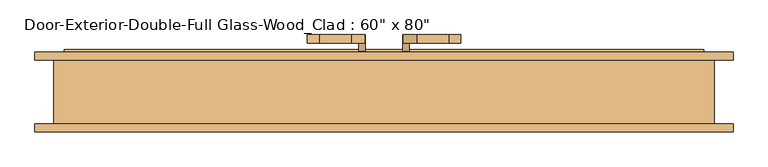
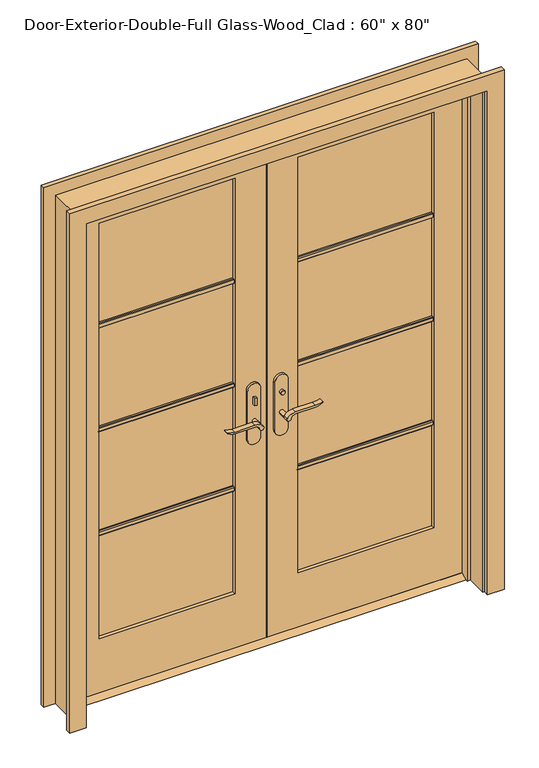
"""IFC4 building model written with IfcOpenShell, lengths in millimetres: door geometry."""

from ifc_helpers import new_model, si_unit, point, frame, frame_2d, origin, place, context, project, spatial, polyline, circle_curve, trimmed, segment, composite_curve, outline, extrude, faceted_brep, source, transform, mapped, element, save


def door_94998e6c(model_context):
    return source(origin(), model_context, "Body", "SolidModel", [
        extrude(outline(polyline([(38.1, 12.7), (73.025, 12.7), (98.425, 0.0), (12.7, 0.0), (38.1, 12.7)])), frame((-762.0, 0.0, 0.0), z_axis=(1.0, 0.0, 0.0), x_axis=(0.0, 1.0, 0.0)), (0.0, 0.0, 1.0), 1524.0),
        extrude(outline(polyline([(-47.4019111, 18.1), (-57.4019111, 18.1), (-57.4019111, 28.1), (-47.4019111, 28.1), (-47.4019111, 18.1)])), frame((0.0, 0.0, 981.9), z_axis=(0.0, 0.0, 1.0), x_axis=(1.0, 0.0, 0.0)), (0.0, 0.0, 1.0), 30.0),
        extrude(outline(composite_curve([segment(trimmed(circle_curve(frame_2d((996.9, -52.4019111)), 8.0), [point((996.9, -60.4019111))], [point((996.9, -44.4019111))], False, "CARTESIAN"), True, "CONTINUOUS"), segment(trimmed(circle_curve(frame_2d((996.9, -52.4019111)), 8.0), [point((996.9, -44.4019111))], [point((996.9, -60.4019111))], False, "CARTESIAN"), True, "CONTINUOUS")], self_intersect=False)), frame((0.0, 83.025, 0.0), z_axis=(0.0, 1.0, 0.0), x_axis=(0.0, 0.0, 1.0)), (0.0, 0.0, 1.0), 10.0),
        extrude(outline(composite_curve([segment(trimmed(circle_curve(frame_2d((897.1555521, -76.0694241)), 37.2832219), [point((919.0523287, -45.8937749))], [point((934.4, -77.7693445))], False, "CARTESIAN"), True, "CONTINUOUS"), segment(polyline([(934.4, -77.7693445), (934.4, -154.045502)]), True, "CONTINUOUS"), segment(trimmed(circle_curve(frame_2d((1017.6850638, -153.9791202)), 83.2850902), [point((934.4, -154.045502))], [point((939.4, -182.4019111))], True, "CARTESIAN"), True, "CONTINUOUS"), segment(polyline([(939.4, -182.4019111), (936.6135558, -182.4019111)]), True, "CONTINUOUS"), segment(trimmed(circle_curve(frame_2d((986.6709207, -150.4622499)), 59.3791355), [point((936.6135558, -182.4019111))], [point((927.4, -154.045502))], False, "CARTESIAN"), True, "CONTINUOUS"), segment(polyline([(927.4, -154.045502), (927.4, -77.7881013)]), True, "CONTINUOUS"), segment(trimmed(circle_curve(frame_2d((909.2738613, -77.7881013)), 18.1261387), [point((927.4, -77.7881013))], [point((914.4, -60.4019111))], True, "CARTESIAN"), True, "CONTINUOUS"), segment(trimmed(circle_curve(frame_2d((914.4, -52.4019111)), 8.0), [point((914.4, -60.4019111))], [point((919.0523287, -45.8937749))], False, "CARTESIAN"), True, "CONTINUOUS")], self_intersect=False)), frame((0.0, -21.9, 0.0), z_axis=(0.0, 1.0, 0.0), x_axis=(0.0, 0.0, 1.0)), (0.0, 0.0, 1.0), 20.0),
        extrude(outline(composite_curve([segment(trimmed(circle_curve(frame_2d((914.4, -52.4019111)), 8.0), [point((914.3999903, -60.4019111))], [point((919.0523287, -45.8937749))], False, "CARTESIAN"), True, "CONTINUOUS"), segment(trimmed(circle_curve(frame_2d((897.1555521, -76.0694241)), 37.2832219), [point((919.0523287, -45.8937749))], [point((934.4, -77.7693445))], False, "CARTESIAN"), True, "CONTINUOUS"), segment(polyline([(934.4, -77.7693445), (934.4, -154.045502)]), True, "CONTINUOUS"), segment(trimmed(circle_curve(frame_2d((1017.6850638, -153.9791202)), 83.2850902), [point((934.4, -154.045502))], [point((939.4, -182.4019111))], True, "CARTESIAN"), True, "CONTINUOUS"), segment(polyline([(939.4, -182.4019111), (936.6135558, -182.4019111)]), True, "CONTINUOUS"), segment(trimmed(circle_curve(frame_2d((986.6709207, -150.4622499)), 59.3791355), [point((936.6135558, -182.4019111))], [point((927.4, -154.045502))], False, "CARTESIAN"), True, "CONTINUOUS"), segment(polyline([(927.4, -154.045502), (927.4, -77.788099)]), True, "CONTINUOUS"), segment(trimmed(circle_curve(frame_2d((909.2738682, -77.788099)), 18.1261318), [point((927.4, -77.788099))], [point((914.3999903, -60.4019111))], True, "CARTESIAN"), True, "CONTINUOUS")], self_intersect=False)), frame((0.0, 113.025, 0.0), z_axis=(0.0, 1.0, 0.0), x_axis=(0.0, 0.0, 1.0)), (0.0, 0.0, 1.0), 20.0),
        extrude(outline(composite_curve([segment(trimmed(circle_curve(frame_2d((914.4, -52.4019111)), 8.0), [point((914.4, -60.4019111))], [point((914.4, -44.4019111))], False, "CARTESIAN"), True, "CONTINUOUS"), segment(trimmed(circle_curve(frame_2d((914.4, -52.4019111)), 8.0), [point((914.4, -44.4019111))], [point((914.4, -60.4019111))], False, "CARTESIAN"), True, "CONTINUOUS")], self_intersect=False)), frame((0.0, -1.9, 0.0), z_axis=(0.0, 1.0, 0.0), x_axis=(0.0, 0.0, 1.0)), (0.0, 0.0, 1.0), 30.0),
        extrude(outline(composite_curve([segment(trimmed(circle_curve(frame_2d((914.4, -52.4019111)), 8.0), [point((914.4, -60.4019111))], [point((914.4, -44.4019111))], False, "CARTESIAN"), True, "CONTINUOUS"), segment(trimmed(circle_curve(frame_2d((914.4, -52.4019111)), 8.0), [point((914.4, -44.4019111))], [point((914.4, -60.4019111))], False, "CARTESIAN"), True, "CONTINUOUS")], self_intersect=False)), frame((0.0, 83.025, 0.0), z_axis=(0.0, 1.0, 0.0), x_axis=(0.0, 0.0, 1.0)), (0.0, 0.0, 1.0), 30.0),
        extrude(outline(composite_curve([segment(polyline([(844.4, -27.4019111), (1039.4, -27.4019111)]), True, "CONTINUOUS"), segment(trimmed(circle_curve(frame_2d((1039.4, -52.4019111)), 25.0), [point((1039.4, -27.4019111))], [point((1039.4, -77.4019111))], False, "CARTESIAN"), True, "CONTINUOUS"), segment(polyline([(1039.4, -77.4019111), (844.4, -77.4019111)]), True, "CONTINUOUS"), segment(trimmed(circle_curve(frame_2d((844.4, -52.4019111)), 25.0), [point((844.4, -77.4019111))], [point((844.4, -27.4019111))], False, "CARTESIAN"), True, "CONTINUOUS")], self_intersect=False)), frame((0.0, 28.1, 0.0), z_axis=(0.0, 1.0, 0.0), x_axis=(0.0, 0.0, 1.0)), (0.0, 0.0, 1.0), 10.0),
        extrude(outline(composite_curve([segment(polyline([(844.4, -27.4019111), (1039.4, -27.4019111)]), True, "CONTINUOUS"), segment(trimmed(circle_curve(frame_2d((1039.4, -52.4019111)), 25.0), [point((1039.4, -27.4019111))], [point((1039.4, -77.4019111))], False, "CARTESIAN"), True, "CONTINUOUS"), segment(polyline([(1039.4, -77.4019111), (844.4, -77.4019111)]), True, "CONTINUOUS"), segment(trimmed(circle_curve(frame_2d((844.4, -52.4019111)), 25.0), [point((844.4, -77.4019111))], [point((844.4, -27.4019111))], False, "CARTESIAN"), True, "CONTINUOUS")], self_intersect=False)), frame((0.0, 73.025, 0.0), z_axis=(0.0, 1.0, 0.0), x_axis=(0.0, 0.0, 1.0)), (0.0, 0.0, 1.0), 10.0),
        extrude(outline(polyline([(47.3875, 93.025), (57.3875, 93.025), (57.3875, 83.025), (47.3875, 83.025), (47.3875, 93.025)])), frame((0.0, 0.0, 981.9), z_axis=(0.0, 0.0, 1.0), x_axis=(1.0, 0.0, 0.0)), (0.0, 0.0, 1.0), 30.0),
        extrude(outline(composite_curve([segment(trimmed(circle_curve(frame_2d((996.9, 52.3875)), 8.0), [point((996.9, 60.3875))], [point((996.9, 44.3875))], False, "CARTESIAN"), True, "CONTINUOUS"), segment(trimmed(circle_curve(frame_2d((996.9, 52.3875)), 8.0), [point((996.9, 44.3875))], [point((996.9, 60.3875))], False, "CARTESIAN"), True, "CONTINUOUS")], self_intersect=False)), frame((0.0, 18.1, 0.0), z_axis=(0.0, 1.0, 0.0), x_axis=(0.0, 0.0, 1.0)), (0.0, 0.0, 1.0), 10.0),
        extrude(outline(composite_curve([segment(trimmed(circle_curve(frame_2d((914.4, 52.3875)), 8.0), [point((919.0523287, 45.8793637))], [point((914.4, 60.3875))], False, "CARTESIAN"), True, "CONTINUOUS"), segment(trimmed(circle_curve(frame_2d((909.2738613, 77.7736901)), 18.1261387), [point((914.4, 60.3875))], [point((927.4, 77.7736901))], True, "CARTESIAN"), True, "CONTINUOUS"), segment(polyline([(927.4, 77.7736901), (927.4, 154.0310909)]), True, "CONTINUOUS"), segment(trimmed(circle_curve(frame_2d((986.6709207, 150.4478388)), 59.3791355), [point((927.4, 154.0310909))], [point((936.6135558, 182.3875))], False, "CARTESIAN"), True, "CONTINUOUS"), segment(polyline([(936.6135558, 182.3875), (939.4, 182.3875)]), True, "CONTINUOUS"), segment(trimmed(circle_curve(frame_2d((1017.6850638, 153.9647091)), 83.2850902), [point((939.4, 182.3875))], [point((934.4, 154.0310909))], True, "CARTESIAN"), True, "CONTINUOUS"), segment(polyline([(934.4, 154.0310909), (934.4, 77.7549333)]), True, "CONTINUOUS"), segment(trimmed(circle_curve(frame_2d((897.1555521, 76.0550129)), 37.2832219), [point((934.4, 77.7549333))], [point((919.0523287, 45.8793637))], False, "CARTESIAN"), True, "CONTINUOUS")], self_intersect=False)), frame((0.0, 113.025, 0.0), z_axis=(0.0, 1.0, 0.0), x_axis=(0.0, 0.0, 1.0)), (0.0, 0.0, 1.0), 20.0),
        extrude(outline(composite_curve([segment(trimmed(circle_curve(frame_2d((909.2738682, 77.7736878)), 18.1261318), [point((914.3999903, 60.3875))], [point((927.4, 77.7736878))], True, "CARTESIAN"), True, "CONTINUOUS"), segment(polyline([(927.4, 77.7736878), (927.4, 154.0310909)]), True, "CONTINUOUS"), segment(trimmed(circle_curve(frame_2d((986.6709207, 150.4478388)), 59.3791355), [point((927.4, 154.0310909))], [point((936.6135558, 182.3875))], False, "CARTESIAN"), True, "CONTINUOUS"), segment(polyline([(936.6135558, 182.3875), (939.4, 182.3875)]), True, "CONTINUOUS"), segment(trimmed(circle_curve(frame_2d((1017.6850638, 153.9647091)), 83.2850902), [point((939.4, 182.3875))], [point((934.4, 154.0310909))], True, "CARTESIAN"), True, "CONTINUOUS"), segment(polyline([(934.4, 154.0310909), (934.4, 77.7549333)]), True, "CONTINUOUS"), segment(trimmed(circle_curve(frame_2d((897.1555521, 76.0550129)), 37.2832219), [point((934.4, 77.7549333))], [point((919.0523287, 45.8793637))], False, "CARTESIAN"), True, "CONTINUOUS"), segment(trimmed(circle_curve(frame_2d((914.4, 52.3875)), 8.0), [point((919.0523287, 45.8793637))], [point((914.3999903, 60.3875))], False, "CARTESIAN"), True, "CONTINUOUS")], self_intersect=False)), frame((0.0, -21.9, 0.0), z_axis=(0.0, 1.0, 0.0), x_axis=(0.0, 0.0, 1.0)), (0.0, 0.0, 1.0), 20.0),
        extrude(outline(composite_curve([segment(trimmed(circle_curve(frame_2d((914.4, 52.3875)), 8.0), [point((914.4, 60.3875))], [point((914.4, 44.3875))], False, "CARTESIAN"), True, "CONTINUOUS"), segment(trimmed(circle_curve(frame_2d((914.4, 52.3875)), 8.0), [point((914.4, 44.3875))], [point((914.4, 60.3875))], False, "CARTESIAN"), True, "CONTINUOUS")], self_intersect=False)), frame((0.0, 83.025, 0.0), z_axis=(0.0, 1.0, 0.0), x_axis=(0.0, 0.0, 1.0)), (0.0, 0.0, 1.0), 30.0),
        extrude(outline(composite_curve([segment(trimmed(circle_curve(frame_2d((914.4, 52.3875)), 8.0), [point((914.4, 60.3875))], [point((914.4, 44.3875))], False, "CARTESIAN"), True, "CONTINUOUS"), segment(trimmed(circle_curve(frame_2d((914.4, 52.3875)), 8.0), [point((914.4, 44.3875))], [point((914.4, 60.3875))], False, "CARTESIAN"), True, "CONTINUOUS")], self_intersect=False)), frame((0.0, -1.9, 0.0), z_axis=(0.0, 1.0, 0.0), x_axis=(0.0, 0.0, 1.0)), (0.0, 0.0, 1.0), 30.0),
        extrude(outline(composite_curve([segment(trimmed(circle_curve(frame_2d((844.4, 52.3875)), 25.0), [point((844.4, 27.3875))], [point((844.4, 77.3875))], False, "CARTESIAN"), True, "CONTINUOUS"), segment(polyline([(844.4, 77.3875), (1039.4, 77.3875)]), True, "CONTINUOUS"), segment(trimmed(circle_curve(frame_2d((1039.4, 52.3875)), 25.0), [point((1039.4, 77.3875))], [point((1039.4, 27.3875))], False, "CARTESIAN"), True, "CONTINUOUS"), segment(polyline([(1039.4, 27.3875), (844.4, 27.3875)]), True, "CONTINUOUS")], self_intersect=False)), frame((0.0, 73.025, 0.0), z_axis=(0.0, 1.0, 0.0), x_axis=(0.0, 0.0, 1.0)), (0.0, 0.0, 1.0), 10.0),
        extrude(outline(composite_curve([segment(trimmed(circle_curve(frame_2d((844.4, 52.3875)), 25.0), [point((844.4, 27.3875))], [point((844.4, 77.3875))], False, "CARTESIAN"), True, "CONTINUOUS"), segment(polyline([(844.4, 77.3875), (1039.4, 77.3875)]), True, "CONTINUOUS"), segment(trimmed(circle_curve(frame_2d((1039.4, 52.3875)), 25.0), [point((1039.4, 77.3875))], [point((1039.4, 27.3875))], False, "CARTESIAN"), True, "CONTINUOUS"), segment(polyline([(1039.4, 27.3875), (844.4, 27.3875)]), True, "CONTINUOUS")], self_intersect=False)), frame((0.0, 28.1, 0.0), z_axis=(0.0, 1.0, 0.0), x_axis=(0.0, 0.0, 1.0)), (0.0, 0.0, 1.0), 10.0),
        extrude(outline(polyline([(52.07, 1502.171875), (52.07, 1483.121875), (45.72, 1483.121875), (42.545, 1486.296875), (42.545, 1498.996875), (45.72, 1502.171875), (52.07, 1502.171875)])), frame((120.65, 0.0, 0.0), z_axis=(1.0, 0.0, 0.0), x_axis=(0.0, 1.0, 0.0)), (0.0, 0.0, 1.0), 520.7),
        extrude(outline(polyline([(52.07, 1081.88125), (52.07, 1062.83125), (45.72, 1062.83125), (42.545, 1066.00625), (42.545, 1078.70625), (45.72, 1081.88125), (52.07, 1081.88125)])), frame((120.65, 0.0, 0.0), z_axis=(1.0, 0.0, 0.0), x_axis=(0.0, 1.0, 0.0)), (0.0, 0.0, 1.0), 520.7),
        extrude(outline(polyline([(52.07, 661.590625), (52.07, 642.540625), (45.72, 642.540625), (42.545, 645.715625), (42.545, 658.415625), (45.72, 661.590625), (52.07, 661.590625)])), frame((120.65, 0.0, 0.0), z_axis=(1.0, 0.0, 0.0), x_axis=(0.0, 1.0, 0.0)), (0.0, 0.0, 1.0), 520.7),
        extrude(outline(polyline([(59.055, 1502.171875), (65.405, 1502.171875), (68.58, 1498.996875), (68.58, 1486.296875), (65.405, 1483.121875), (59.055, 1483.121875), (59.055, 1502.171875)])), frame((-641.35, 0.0, 0.0), z_axis=(1.0, 0.0, 0.0), x_axis=(0.0, 1.0, 0.0)), (0.0, 0.0, 1.0), 520.7),
        extrude(outline(polyline([(59.055, 1081.88125), (65.405, 1081.88125), (68.58, 1078.70625), (68.58, 1066.00625), (65.405, 1062.83125), (59.055, 1062.83125), (59.055, 1081.88125)])), frame((-641.35, 0.0, 0.0), z_axis=(1.0, 0.0, 0.0), x_axis=(0.0, 1.0, 0.0)), (0.0, 0.0, 1.0), 520.7),
        extrude(outline(polyline([(59.055, 661.590625), (65.405, 661.590625), (68.58, 658.415625), (68.58, 645.715625), (65.405, 642.540625), (59.055, 642.540625), (59.055, 661.590625)])), frame((-641.35, 0.0, 0.0), z_axis=(1.0, 0.0, 0.0), x_axis=(0.0, 1.0, 0.0)), (0.0, 0.0, 1.0), 520.7),
        extrude(outline(polyline([(59.055, 1502.171875), (65.405, 1502.171875), (68.58, 1498.996875), (68.58, 1486.296875), (65.405, 1483.121875), (59.055, 1483.121875), (59.055, 1502.171875)])), frame((120.65, 0.0, 0.0), z_axis=(1.0, 0.0, 0.0), x_axis=(0.0, 1.0, 0.0)), (0.0, 0.0, 1.0), 520.7),
        extrude(outline(polyline([(59.055, 1081.88125), (65.405, 1081.88125), (68.58, 1078.70625), (68.58, 1066.00625), (65.405, 1062.83125), (59.055, 1062.83125), (59.055, 1081.88125)])), frame((120.65, 0.0, 0.0), z_axis=(1.0, 0.0, 0.0), x_axis=(0.0, 1.0, 0.0)), (0.0, 0.0, 1.0), 520.7),
        extrude(outline(polyline([(59.055, 661.590625), (65.405, 661.590625), (68.58, 658.415625), (68.58, 645.715625), (65.405, 642.540625), (59.055, 642.540625), (59.055, 661.590625)])), frame((120.65, 0.0, 0.0), z_axis=(1.0, 0.0, 0.0), x_axis=(0.0, 1.0, 0.0)), (0.0, 0.0, 1.0), 520.7),
        extrude(outline(polyline([(52.07, 1502.171875), (52.07, 1483.121875), (45.72, 1483.121875), (42.545, 1486.296875), (42.545, 1498.996875), (45.72, 1502.171875), (52.07, 1502.171875)])), frame((-641.35, 0.0, 0.0), z_axis=(1.0, 0.0, 0.0), x_axis=(0.0, 1.0, 0.0)), (0.0, 0.0, 1.0), 520.7),
        extrude(outline(polyline([(52.07, 1081.88125), (52.07, 1062.83125), (45.72, 1062.83125), (42.545, 1066.00625), (42.545, 1078.70625), (45.72, 1081.88125), (52.07, 1081.88125)])), frame((-641.35, 0.0, 0.0), z_axis=(1.0, 0.0, 0.0), x_axis=(0.0, 1.0, 0.0)), (0.0, 0.0, 1.0), 520.7),
        extrude(outline(polyline([(52.07, 661.590625), (52.07, 642.540625), (45.72, 642.540625), (42.545, 645.715625), (42.545, 658.415625), (45.72, 661.590625), (52.07, 661.590625)])), frame((-641.35, 0.0, 0.0), z_axis=(1.0, 0.0, 0.0), x_axis=(0.0, 1.0, 0.0)), (0.0, 0.0, 1.0), 520.7),
        extrude(outline(polyline([(0.0, 768.35), (0.0, 831.85), (2101.85, 831.85), (2101.85, -831.85), (0.0, -831.85), (0.0, -768.35), (2038.35, -768.35), (2038.35, 768.35), (0.0, 768.35)])), frame((0.0, 73.025, 0.0), z_axis=(0.0, 1.0, 0.0), x_axis=(0.0, 0.0, 1.0)), (0.0, 0.0, 1.0), 19.05),
        extrude(outline(polyline([(0.0, 768.35), (0.0, 831.85), (2101.85, 831.85), (2101.85, -831.85), (0.0, -831.85), (0.0, -768.35), (2038.35, -768.35), (2038.35, 768.35), (0.0, 768.35)])), frame((0.0, -98.425, 0.0), z_axis=(0.0, 1.0, 0.0), x_axis=(0.0, 0.0, 1.0)), (0.0, 0.0, 1.0), 19.05),
        extrude(outline(polyline([(12.7, 762.0), (2032.0, 762.0), (2032.0, 1.5875), (12.7, 1.5875), (12.7, 762.0)]), holes=[polyline([(1912.9375, 120.65), (1912.9375, 641.35), (231.775, 641.35), (231.775, 120.65), (1912.9375, 120.65)])]), frame((0.0, 38.1, 0.0), z_axis=(0.0, 1.0, 0.0), x_axis=(0.0, 0.0, 1.0)), (0.0, 0.0, 1.0), 34.925),
        extrude(outline(polyline([(2032.0, -762.0), (12.7, -762.0), (12.7, -1.6019111), (2032.0, -1.6019111), (2032.0, -762.0)]), holes=[polyline([(231.775, -641.35), (1912.9375, -641.35), (1912.9375, -120.65), (231.775, -120.65), (231.775, -641.35)])]), frame((0.0, 38.1, 0.0), z_axis=(0.0, 1.0, 0.0), x_axis=(0.0, 0.0, 1.0)), (0.0, 0.0, 1.0), 34.925),
        faceted_brep([(787.4, 73.025, 0.0), (787.4, -79.375, 0.0), (762.0, -79.375, 0.0), (762.0, 3.175, 0.0), (749.3, 3.175, 0.0), (749.3, 38.1, 0.0), (762.0, 38.1, 0.0), (762.0, 73.025, 0.0), (787.4, 73.025, 2057.4), (787.4, -79.375, 2057.4), (-787.4, -79.375, 2057.4), (-787.4, -79.375, 0.0), (-762.0, -79.375, 0.0), (-762.0, -79.375, 2032.0), (762.0, -79.375, 2032.0), (762.0, 3.175, 2032.0), (-762.0, 3.175, 2032.0), (-762.0, 3.175, 0.0), (-749.3, 3.175, 0.0), (-749.3, 3.175, 2019.3), (749.3, 3.175, 2019.3), (749.3, 38.1, 2019.3), (1.5875, 38.1, 2019.3), (-1.6019111, 38.1, 2019.3), (-749.3, 38.1, 2019.3), (-749.3, 38.1, 0.0), (-762.0, 38.1, 0.0), (-762.0, 38.1, 2032.0), (-1.6019111, 38.1, 2032.0), (1.5875, 38.1, 2032.0), (762.0, 38.1, 2032.0), (762.0, 73.025, 2032.0), (1.5875, 73.025, 2032.0), (-1.6019111, 73.025, 2032.0), (-762.0, 73.025, 2032.0), (-762.0, 73.025, 0.0), (-787.4, 73.025, 0.0), (-787.4, 73.025, 2057.4)], [[[0, 1, 2, 3, 4, 5, 6, 7]], [[1, 0, 8, 9]], [[2, 1, 9, 10, 11, 12, 13, 14]], [[3, 2, 14, 15]], [[4, 3, 15, 16, 17, 18, 19, 20]], [[5, 4, 20, 21]], [[6, 5, 21, 22, 23, 24, 25, 26, 27, 28, 29, 30]], [[7, 6, 30, 31]], [[0, 7, 31, 32, 33, 34, 35, 36, 37, 8]], [[9, 8, 37, 10]], [[14, 13, 16, 15]], [[20, 19, 24, 23, 22, 21]], [[31, 30, 29, 28, 27, 34, 33, 32]], [[12, 11, 36, 35, 26, 25, 18, 17]], [[11, 10, 37, 36]], [[13, 12, 17, 16]], [[19, 18, 25, 24]], [[27, 26, 35, 34]]]),
        extrude(outline(polyline([(641.35, 52.07), (120.65, 52.07), (120.65, 59.055), (641.35, 59.055), (641.35, 52.07)])), frame((0.0, 0.0, 231.775), z_axis=(0.0, 0.0, 1.0), x_axis=(1.0, 0.0, 0.0)), (0.0, 0.0, 1.0), 1681.1625),
        extrude(outline(polyline([(-120.65, 52.07), (-641.35, 52.07), (-641.35, 59.055), (-120.65, 59.055), (-120.65, 52.07)])), frame((0.0, 0.0, 231.775), z_axis=(0.0, 0.0, 1.0), x_axis=(1.0, 0.0, 0.0)), (0.0, 0.0, 1.0), 1681.1625),
    ])


if __name__ == "__main__":
    model = new_model("IFC4")
    model_context = context("Model", 3, world=origin())
    ifc_project = project(units=[si_unit("LENGTHUNIT", "METRE", prefix="MILLI")], contexts=[model_context])
    site = spatial("IfcSite", under=ifc_project)
    building = spatial("IfcBuilding", under=site)
    placement = place(None, origin())
    door_shape = door_94998e6c(model_context)
    element("IfcDoor", 1, ObjectType="Door-Exterior-Double-Full Glass-Wood_Clad : 60\" x 80\"", at=placement, inside=building, context=model_context, shape_type="MappedRepresentation", body=[
        mapped(door_shape, transform((0.0, 0.0, 0.0), x_axis=(1.0, 0.0, 0.0), y_axis=(0.0, 1.0, 0.0), z_axis=(0.0, 0.0, 1.0))),
    ])
    save(model, "model.ifc")

# Revit data of these elements
# Type "Door-Exterior-Double-Full Glass-Wood_Clad : 60\" x 80\""
#   Type Mark = "8"
#   Assembly Code = "B2030100"
#   Analytic Construction = "French door, wood frame with double glass"
#   Top Rail = 0' - 4 11/16"
#   Threshold Offset [instance default] = 0' - 0 1/2"
#   Thickness = 0' - 1 3/8"
#   Thermal Resistance (R) = 1.9158 (h·ft²·°F)/BTU
#   Swing Angle [instance default] = 90.00°
#   Stiles = 0' - 4 3/4"
#   Rough Width = 5' - 2"
#   Rough Height = 6' - 9"
#   Panel Width = 2' - 6"
#   Door Offset [instance default] = 0' - 0"
#   Height = 6' - 8"
#   Width = 5' - 0"
#   Heat Transfer Coefficient (U) = 0.5220 BTU/(h·ft²·°F)
#   Bottom Rail = 0' - 9 1/8"
#   Exterior Trim [instance default] = yes
#   Threshold [instance default] = yes
#   Show Grill [instance default] = yes
#   Function = 1
#   Trim Material = Cherry
#   Threshold Material = Cherry
#   Panel Material = Cherry
#   Glazing = Glass
#   Frame Material = Cherry
#   Door Handle Material = Aluminum
#   Visual Light Transmittance = 0
#   Solar Heat Gain Coefficient = 0
#   Wall Closure = (empty or 0)
#   Construction Type = (empty or 0)
# Element 1 (IfcDoor, "Door-Exterior-Double-Full Glass-Wood_Clad : 60\" x 80\"")
#   Materials on its faces: "Cherry", "Aluminum", "Glass"
# Materials
#   "Cherry": class "Wood", colour RGB 226 177 128, transparency 0, Description = "Prunus Serotina", Cost = 0
#   "Glass": class "Glass", colour RGB 0 128 192, transparency 0.75, Description = "Soda Lime Glass", Cost = 0
#   "Aluminum": class "Metal", colour RGB 247 247 247, transparency 0, Description = "Aluminum 6061", Cost = 0
